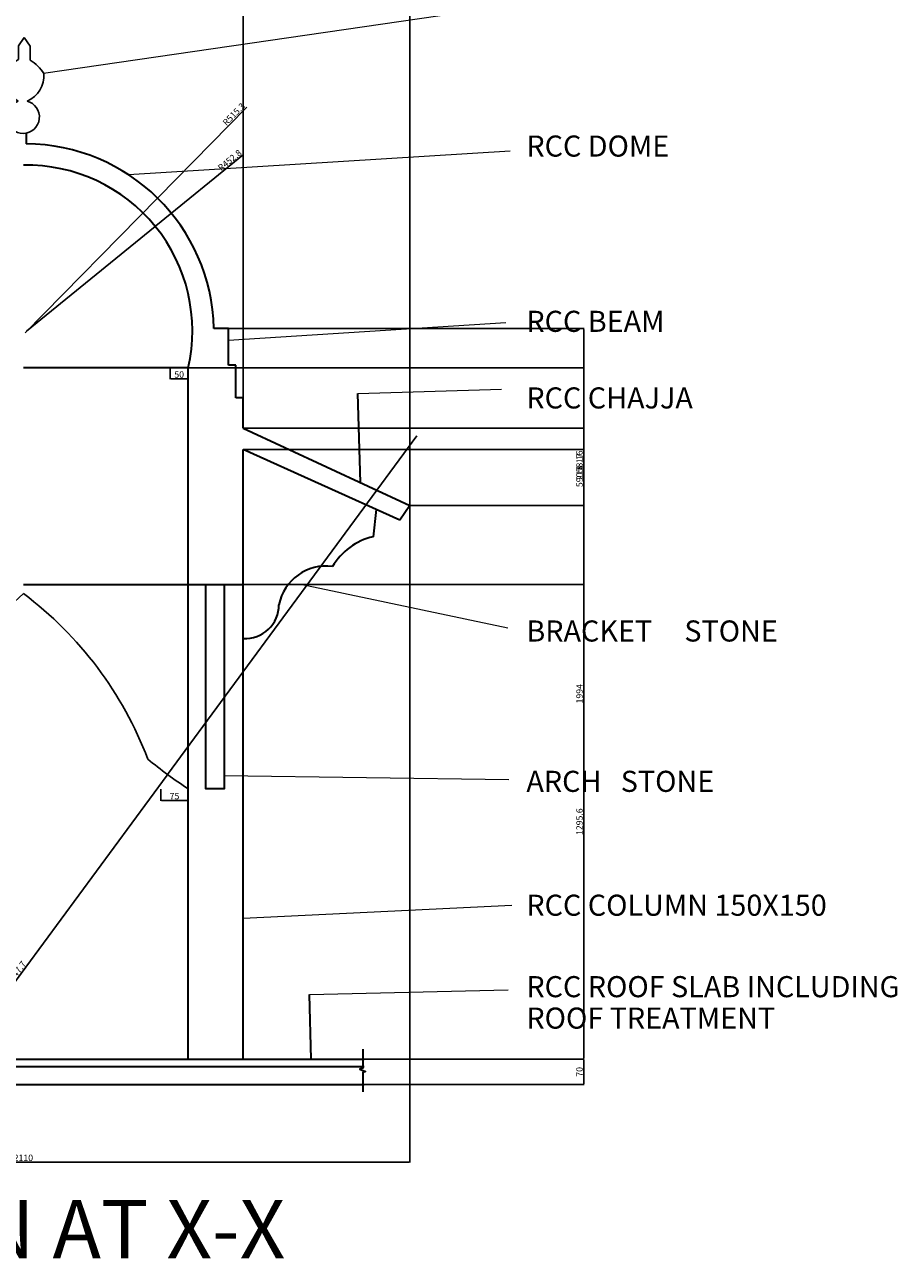
# Model space of a CAD drawing. Units: millimetres. Extents: x 498 to 8860, y -426 to 8717.
# Tile 6 of 9: x 1798 to 4180, y 3606 to 6976. Entities that reach past the tile are written whole.
import ezdxf

# ---------------------------------------------------------------- set-up
doc = ezdxf.new("R2010")
doc.units = ezdxf.units.MM
for name, color, linetype, lineweight in [('A-ANNO-DIMS', 2, 'Continuous', 18), ('A-ANNO-TEXT', 3, 'Continuous', 18), ('A-DETL', 7, 'Continuous', 25), ('A-SECT', 7, 'Continuous', 35)]:
    doc.layers.add(name, color=color, linetype=linetype, lineweight=lineweight)
doc.styles.get("Standard").update_dxf_attribs({"font": 'arial.ttf'})
doc.dimstyles.new('ISO-25', dxfattribs={"dimtxt": 17.5, "dimasz": 2.5, "dimexe": 1.25, "dimexo": 0.625, "dimtad": 1, "dimdec": 0, "dimtxsty": 'Standard', "dimcen": 2.5, "dimadec": 0, "dimazin": 0, "dimtfac": 1, "dimtdec": 0, "dimtmove": 0, "dimatfit": 3, "dimfxl": 1, "dimarcsym": 0})

# ---------------------------------------------------------------- blocks, each defined once
blk = doc.blocks.new('*D30')
at = {"layer": 'A-ANNO-DIMS', "color": 0, "lineweight": -2, "transparency": 16777216}
for p, q in [((2195, 6038.9), (2195, 6008.7)), ((2244.7, 6038.9), (2244.7, 6008.7)), ((2242.2, 6010), (2197.5, 6010))]:
    blk.add_line(p, q, dxfattribs=at)
at = {"layer": 'A-ANNO-DIMS', "color": 0, "transparency": 16777216}
for points in [[(2197.5, 6010.4), (2197.5, 6009.6), (2195, 6010)], [(2242.2, 6010.4), (2242.2, 6009.6), (2244.7, 6010)]]:
    blk.add_solid(points, dxfattribs=at)
at = {"layer": 'Defpoints', "color": 0, "transparency": 16777216}
for p in [(2195, 6039.5), (2244.7, 6039.5), (2195, 6010)]:
    blk.add_point(p, dxfattribs=at)
at = {"layer": 'A-ANNO-DIMS', "color": 0, "transparency": 16777216, "insert": (2219.9, 6019.5), "char_height": 17.5, "attachment_point": 5}
blk.add_mtext('50', dxfattribs=at)
blk = doc.blocks.new('*D33')
at = {"layer": 'A-ANNO-DIMS', "color": 0, "lineweight": -2, "transparency": 16777216}
for p, q in [((2169.5, 4890.1), (2169.5, 4857.7)), ((2244.7, 4889.9), (2244.7, 4857.7)), ((2242.2, 4858.9), (2172, 4858.9))]:
    blk.add_line(p, q, dxfattribs=at)
at = {"layer": 'A-ANNO-DIMS', "color": 0, "transparency": 16777216}
for points in [[(2172, 4859.3), (2172, 4858.5), (2169.5, 4858.9)], [(2242.2, 4859.3), (2242.2, 4858.5), (2244.7, 4858.9)]]:
    blk.add_solid(points, dxfattribs=at)
at = {"layer": 'Defpoints', "color": 0, "transparency": 16777216}
for p in [(2169.5, 4890.7), (2244.7, 4890.6), (2169.5, 4858.9)]:
    blk.add_point(p, dxfattribs=at)
at = {"layer": 'A-ANNO-DIMS', "color": 0, "transparency": 16777216, "insert": (2207.1, 4868.4), "char_height": 17.5, "attachment_point": 5}
blk.add_mtext('75', dxfattribs=at)
blk = doc.blocks.new('FINIAL-BRASS')
for p, q in [((41.3, 239), (57, 261.6)), ((41.3, 202), (41.3, 239)), ((57, 261.6), (73.3, 238.5)), ((73.3, 199.9), (73.3, 238.5))]:
    blk.add_line(p, q)
for centre, radius, start, end in [((108.5, 89), 131.5, 120.7656, 145.5289), ((18.2, 106.2), 108.7, 31.7357, 59.5088), ((81.5, 158.5), 81.5, 176.5528, 239.9655), ((34.6, 158.5), 76.2, 293.2182, 3.7332), ((53.5, 44.9), 44.9, 106.5437, 75.6662)]:
    blk.add_arc(centre, radius, start, end)
blk = doc.blocks.new('BRACKET-STONE')
for centre, radius, start, end in [((1183.8, -291.1), 1104.6, 131.6209, 159.0769), ((-158.8, -276), 1013.9, 20.7397, 53.0882), ((-446.2, 819.4), 933, 298.5683, 309.875), ((1523.8, 965), 1147.7, 230.2129, 237.0762)]:
    blk.add_arc(centre, radius, start, end)
blk = doc.blocks.new('*D43')
at = {"layer": 'A-ANNO-DIMS', "color": 0, "lineweight": -2, "transparency": 16777216}
for p, q in [((739.8, 5663.4), (739.8, 3870.5)), ((2849.6, 5663.4), (2849.6, 3870.5)), ((742.3, 3871.8), (2847.1, 3871.8))]:
    blk.add_line(p, q, dxfattribs=at)
at = {"layer": 'A-ANNO-DIMS', "color": 0, "transparency": 16777216}
for points in [[(742.3, 3872.2), (742.3, 3871.3), (739.8, 3871.8)], [(2847.1, 3872.2), (2847.1, 3871.3), (2849.6, 3871.8)]]:
    blk.add_solid(points, dxfattribs=at)
at = {"layer": 'Defpoints', "color": 0, "transparency": 16777216}
for p in [(739.8, 5664), (2849.6, 5664), (2849.6, 3871.8)]:
    blk.add_point(p, dxfattribs=at)
at = {"layer": 'A-ANNO-DIMS', "color": 0, "transparency": 16777216, "insert": (1794.7, 3881.3), "char_height": 17.5, "attachment_point": 5}
blk.add_mtext('2110', dxfattribs=at)
blk = doc.blocks.new('*D45')
at = {"layer": 'A-ANNO-DIMS', "color": 0, "lineweight": -2, "transparency": 16777216}
for p, q in [((2395.4, 5448.8), (3325.4, 5448.8)), ((3324.2, 4155.7), (3324.2, 5446.3)), ((2395.4, 4153.2), (3325.4, 4153.2))]:
    blk.add_line(p, q, dxfattribs=at)
at = {"layer": 'A-ANNO-DIMS', "color": 0, "transparency": 16777216}
for points in [[(3323.8, 5446.3), (3324.6, 5446.3), (3324.2, 5448.8)], [(3323.8, 4155.7), (3324.6, 4155.7), (3324.2, 4153.2)]]:
    blk.add_solid(points, dxfattribs=at)
at = {"layer": 'Defpoints', "color": 0, "transparency": 16777216}
for p in [(2394.7, 5448.8), (3324.2, 5448.8), (2394.7, 4153.2)]:
    blk.add_point(p, dxfattribs=at)
at = {"layer": 'A-ANNO-DIMS', "color": 0, "transparency": 16777216, "insert": (3314.6, 4801), "char_height": 17.5, "attachment_point": 5, "rotation": 90}
blk.add_mtext('1295.6', dxfattribs=at)
blk = doc.blocks.new('*D46')
at = {"layer": 'A-ANNO-DIMS', "color": 0, "lineweight": -2, "transparency": 16777216}
for p, q in [((2245.4, 6039.5), (3325.4, 6039.5)), ((3324.2, 5451.3), (3324.2, 6037)), ((2245.4, 5448.8), (3325.4, 5448.8))]:
    blk.add_line(p, q, dxfattribs=at)
at = {"layer": 'A-ANNO-DIMS', "color": 0, "transparency": 16777216}
for points in [[(3323.8, 6037), (3324.6, 6037), (3324.2, 6039.5)], [(3323.8, 5451.3), (3324.6, 5451.3), (3324.2, 5448.8)]]:
    blk.add_solid(points, dxfattribs=at)
at = {"layer": 'Defpoints', "color": 0, "transparency": 16777216}
for p in [(2244.7, 6039.5), (3324.2, 6039.5), (2244.7, 5448.8)]:
    blk.add_point(p, dxfattribs=at)
at = {"layer": 'A-ANNO-DIMS', "color": 0, "transparency": 16777216, "insert": (3314.6, 5744.1), "char_height": 17.5, "attachment_point": 5, "rotation": 90}
blk.add_mtext('590.8', dxfattribs=at)
blk = doc.blocks.new('*D47')
at = {"layer": 'A-ANNO-DIMS', "color": 0, "lineweight": -2, "transparency": 16777216}
for p, q in [((2315.4, 6147.2), (3325.4, 6147.2)), ((3324.2, 4155.7), (3324.2, 6144.7)), ((2395.4, 4153.2), (3325.4, 4153.2))]:
    blk.add_line(p, q, dxfattribs=at)
at = {"layer": 'A-ANNO-DIMS', "color": 0, "transparency": 16777216}
for points in [[(3323.8, 6144.7), (3324.6, 6144.7), (3324.2, 6147.2)], [(3323.8, 4155.7), (3324.6, 4155.7), (3324.2, 4153.2)]]:
    blk.add_solid(points, dxfattribs=at)
at = {"layer": 'Defpoints', "color": 0, "transparency": 16777216}
for p in [(2314.7, 6147.2), (3324.2, 6147.2), (2394.7, 4153.2)]:
    blk.add_point(p, dxfattribs=at)
at = {"layer": 'A-ANNO-DIMS', "color": 0, "transparency": 16777216, "insert": (3314.6, 5150.2), "char_height": 17.5, "attachment_point": 5, "rotation": 90}
blk.add_mtext('1994', dxfattribs=at)
blk = doc.blocks.new('*D48')
at = {"layer": 'A-ANNO-DIMS', "color": 0, "lineweight": -2, "transparency": 16777216}
for p, q in [((2395.4, 5875.2), (3325.4, 5875.2)), ((3324.2, 5872.7), (3324.2, 5819.5)), ((2395.4, 5817), (3325.4, 5817)), ((3324.2, 5817), (3324.2, 5754.2))]:
    blk.add_line(p, q, dxfattribs=at)
at = {"layer": 'A-ANNO-DIMS', "color": 0, "transparency": 16777216}
for points in [[(3323.8, 5872.7), (3324.6, 5872.7), (3324.2, 5875.2)], [(3323.8, 5819.5), (3324.6, 5819.5), (3324.2, 5817)]]:
    blk.add_solid(points, dxfattribs=at)
at = {"layer": 'Defpoints', "color": 0, "transparency": 16777216}
for p in [(2394.7, 5875.2), (2394.7, 5817), (3324.2, 5817)]:
    blk.add_point(p, dxfattribs=at)
at = {"layer": 'A-ANNO-DIMS', "color": 0, "transparency": 16777216, "insert": (3314.6, 5784.4), "char_height": 17.5, "attachment_point": 5, "rotation": 90}
blk.add_mtext('58.16', dxfattribs=at)
blk = doc.blocks.new('*D49')
at = {"layer": 'A-ANNO-DIMS', "color": 0, "lineweight": -2, "transparency": 16777216}
for p, q in [((2394.7, 5875.8), (2394.7, 7224.4)), ((2397.2, 7223.1), (2847.1, 7223.1)), ((2849.6, 5664.6), (2849.6, 7224.4))]:
    blk.add_line(p, q, dxfattribs=at)
at = {"layer": 'A-ANNO-DIMS', "color": 0, "transparency": 16777216}
for points in [[(2397.2, 7223.5), (2397.2, 7222.7), (2394.7, 7223.1)], [(2847.1, 7223.5), (2847.1, 7222.7), (2849.6, 7223.1)]]:
    blk.add_solid(points, dxfattribs=at)
at = {"layer": 'Defpoints', "color": 0, "transparency": 16777216}
for p in [(2849.6, 7223.1), (2394.7, 5875.2), (2849.6, 5664)]:
    blk.add_point(p, dxfattribs=at)
at = {"layer": 'A-ANNO-DIMS', "color": 0, "transparency": 16777216, "insert": (2622.2, 7232.7), "char_height": 17.5, "attachment_point": 5}
blk.add_mtext('454.9', dxfattribs=at)
blk = doc.blocks.new('*D50')
at = {"layer": 'A-ANNO-DIMS', "color": 0, "lineweight": -2, "transparency": 16777216}
for p, q in [((2395.4, 5875.2), (3325.4, 5875.2)), ((3324.2, 5872.7), (3324.2, 5666.5)), ((2850.3, 5664), (3325.4, 5664))]:
    blk.add_line(p, q, dxfattribs=at)
at = {"layer": 'A-ANNO-DIMS', "color": 0, "transparency": 16777216}
for points in [[(3323.8, 5872.7), (3324.6, 5872.7), (3324.2, 5875.2)], [(3323.8, 5666.5), (3324.6, 5666.5), (3324.2, 5664)]]:
    blk.add_solid(points, dxfattribs=at)
at = {"layer": 'Defpoints', "color": 0, "transparency": 16777216}
for p in [(2394.7, 5875.2), (2849.6, 5664), (3324.2, 5664)]:
    blk.add_point(p, dxfattribs=at)
at = {"layer": 'A-ANNO-DIMS', "color": 0, "transparency": 16777216, "insert": (3314.8, 5769.6), "char_height": 17.5, "attachment_point": 5, "rotation": 90}
blk.add_mtext('211.17', dxfattribs=at)
blk = doc.blocks.new('*D51')
at = {"layer": 'A-ANNO-DIMS', "color": 0, "lineweight": -2, "transparency": 16777216}
for p, q in [((2725.4, 4153.2), (3325.4, 4153.2)), ((3324.2, 4150.7), (3324.2, 4085.7)), ((2725.4, 4083.2), (3325.4, 4083.2))]:
    blk.add_line(p, q, dxfattribs=at)
at = {"layer": 'A-ANNO-DIMS', "color": 0, "transparency": 16777216}
for points in [[(3323.8, 4150.7), (3324.6, 4150.7), (3324.2, 4153.2)], [(3323.8, 4085.7), (3324.6, 4085.7), (3324.2, 4083.2)]]:
    blk.add_solid(points, dxfattribs=at)
at = {"layer": 'Defpoints', "color": 0, "transparency": 16777216}
for p in [(2724.7, 4153.2), (2724.7, 4083.2), (3324.2, 4083.2)]:
    blk.add_point(p, dxfattribs=at)
at = {"layer": 'A-ANNO-DIMS', "color": 0, "transparency": 16777216, "insert": (3314.6, 4118.2), "char_height": 17.5, "attachment_point": 5, "rotation": 90}
blk.add_mtext('70', dxfattribs=at)
blk = doc.blocks.new('*D74')
at = {"layer": 'A-ANNO-DIMS', "color": 0, "lineweight": -2, "transparency": 16777216}
for p, q in [((2404.4, 6751.2), (2162.5, 6505)), ((1799.6, 6135.6), (2160.7, 6503.2))]:
    blk.add_line(p, q, dxfattribs=at)
at = {"layer": 'A-ANNO-DIMS', "color": 0, "transparency": 16777216}
blk.add_solid([(2162.2, 6505.3), (2162.7, 6504.7), (2160.7, 6503.2)], dxfattribs=at)
at = {"layer": 'Defpoints', "color": 0, "transparency": 16777216}
for p in [(2160.7, 6503.2), (1799.6, 6135.6)]:
    blk.add_point(p, dxfattribs=at)
at = {"layer": 'A-ANNO-DIMS', "color": 0, "transparency": 16777216, "insert": (2370.6, 6730.4), "char_height": 17.5, "attachment_point": 5, "rotation": 45.5059}
blk.add_mtext('R515.3', dxfattribs=at)
blk = doc.blocks.new('*D75')
at = {"layer": 'A-ANNO-DIMS', "color": 0, "lineweight": -2, "transparency": 16777216}
for p, q in [((2395.3, 6621.7), (2156.5, 6427.6)), ((1803.3, 6140.3), (2154.6, 6426))]:
    blk.add_line(p, q, dxfattribs=at)
at = {"layer": 'A-ANNO-DIMS', "color": 0, "transparency": 16777216}
blk.add_solid([(2156.3, 6427.9), (2156.8, 6427.3), (2154.6, 6426)], dxfattribs=at)
at = {"layer": 'Defpoints', "color": 0, "transparency": 16777216}
for p in [(2154.6, 6426), (1803.3, 6140.3)]:
    blk.add_point(p, dxfattribs=at)
at = {"layer": 'A-ANNO-DIMS', "color": 0, "transparency": 16777216, "insert": (2359.3, 6604.8), "char_height": 17.5, "attachment_point": 5, "rotation": 39.1178}
blk.add_mtext('R452.8', dxfattribs=at)
blk = doc.blocks.new('*D76')
at = {"layer": 'A-ANNO-DIMS', "color": 0, "lineweight": -2, "transparency": 16777216}
for p, q in [((2868.5, 5853.9), (2188.2, 4929.6)), ((1753.1, 4338.5), (2186.7, 4927.6))]:
    blk.add_line(p, q, dxfattribs=at)
at = {"layer": 'A-ANNO-DIMS', "color": 0, "transparency": 16777216}
blk.add_solid([(2186.4, 4927.8), (2187.1, 4927.3), (2188.2, 4929.6)], dxfattribs=at)
at = {"layer": 'Defpoints', "color": 0, "transparency": 16777216}
for p in [(2868.5, 5853.9), (2188.2, 4929.6)]:
    blk.add_point(p, dxfattribs=at)
at = {"layer": 'A-ANNO-DIMS', "color": 0, "transparency": 16777216, "insert": (1772.4, 4380.6), "char_height": 17.5, "attachment_point": 5, "rotation": 53.6461}
blk.add_mtext('R1147.7', dxfattribs=at)

msp = doc.modelspace()

# ---------------------------------------------------------------- linework, layer by layer
at = {"layer": 'A-ANNO-TEXT'}
for p, q in [((2081.16, 6567.175), (3122.821, 6631.816)), ((2354.726, 6115.745), (3111.023, 6163.21)), ((2707.096, 5969.553), (3099.478, 5981.733)), ((2552.178, 5449.241), (3116.865, 5330.088)), ((2342.353, 4927.161), (3119.838, 4915.994)), ((2394.726, 4538.083), (3127.724, 4573.133)), ((2575.958, 4329.528), (3117.407, 4341.91))]:
    msp.add_line(p, q, dxfattribs=at)
msp.add_lwpolyline([(1849.694, 6844.528), (3132.176, 7031.12)], dxfattribs=at)
at = {"layer": 'A-SECT'}
for p, q in [((1802.162, 6680.333), (1802.162, 6650.916)), ((2354.726, 6147.245), (2314.726, 6147.245)), ((2354.726, 6047.245), (2354.726, 6147.245)), ((2244.726, 6039.541), (1794.726, 6039.541)), ((2244.726, 5448.755), (2244.726, 6039.541)), ((2374.726, 6047.245), (2354.726, 6047.245)), ((2374.726, 5957.887), (2374.726, 6047.245)), ((2714.636, 5726.663), (2707.096, 5969.553)), ((2394.726, 5957.887), (2374.726, 5957.887)), ((2394.726, 5875.163), (2394.726, 5957.887)), ((2394.726, 5875.163), (2849.644, 5663.993)), ((2394.726, 5448.755), (2394.726, 5817.007)), ((2822.299, 5623.74), (2394.726, 5817.007)), ((2849.644, 5663.993), (2822.299, 5623.74)), ((2757.051, 5653.233), (2749.118, 5578.673)), ((1794.726, 5448.755), (2394.726, 5448.755)), ((2244.726, 4153.169), (2244.726, 5448.755)), ((2394.726, 4153.169), (2394.726, 5448.755)), ((2579.991, 4153.169), (2575.958, 4329.528)), ((864.726, 4153.169), (2724.726, 4153.169)), ((864.726, 4133.169), (2724.726, 4133.169)), ((864.726, 4083.169), (2724.726, 4083.169))]:
    msp.add_line(p, q, dxfattribs=at)
msp.add_lwpolyline([(2293.009, 5448.755), (2342.353, 5448.755), (2342.353, 4890.556), (2293.009, 4890.556)], close=True, dxfattribs=at)
msp.add_lwpolyline([(2721.018, 4180.433), (2721.018, 4127.866), (2713.259, 4125.041), (2728.777, 4119.393), (2721.018, 4116.569), (2721.018, 4063.756)], dxfattribs=at)
for centre, radius, start, end in [((1799.566, 6135.632), 515.29, 1.291337, 89.711428), ((1803.318, 6140.339), 452.771, 347.13675, 91.087286), ((2787.134, 5410.667), 172.253, 102.750062, 149.710295), ((2620.732, 5367.687), 131.056, 82.254004, 168.811873), ((2400.225, 5393.116), 91.941, 266.570991, 360)]:
    msp.add_arc(centre, radius, start, end, dxfattribs=at)

# ---------------------------------------------------------------- block references
at = {"layer": 'A-DETL'}
for name, p in [('FINIAL-BRASS', (1740.051, 6679.509)), ('BRACKET-STONE', (1344.726, 4888.954))]:
    msp.add_blockref(name, p, dxfattribs=at)

# ---------------------------------------------------------------- texts
at = {"layer": 'A-ANNO-TEXT'}
for s, height, p in [('RCC DOME', 57.5404, (3167.376, 6616.418)), ('RCC BEAM', 57.5404, (3167.376, 6138.023)), ('RCC CHAJJA', 57.5404, (3167.376, 5928.899)), ('BRACKET     STONE', 57.54038, (3167.376, 5292.736)), ('ARCH   STONE', 57.54038, (3167.376, 4882.363)), ('RCC COLUMN 150X150 ', 57.54038, (3167.376, 4544.23)), ('RCC ROOF SLAB INCLUDING', 57.54038, (3167.376, 4321.904)), ('ROOF TREATMENT', 57.54038, (3167.376, 4236.094)), ('SECTION AT X-X', 159.20004, (917.853, 3609.29))]:
    msp.add_text(s, height=height, dxfattribs=at).set_placement(p)

# ---------------------------------------------------------------- dimensions: what is measured, and where the dimension line sits
at = {"layer": 'A-ANNO-DIMS'}
for base, p1, p2, override, picture, middle in [((2849.644, 7223.12), (2394.726, 5875.163), (2849.644, 5663.993), {"dimdec": 1, "dimlfac": 1, "dimrnd": 0, "dimzin": 0, "dimdsep": 46, "dimlunit": 2}, '*D49', (2622.185, 7232.68)), ((2194.985, 6009.99), (2244.726, 6039.541), (2194.985, 6039.541), {"dimclrd": 0, "dimclre": 0, "dimclrt": 0}, '*D30', (2219.855, 6019.55)), ((2849.644, 3871.756), (739.808, 5663.993), (2849.644, 5663.993), {"dimdec": 0, "dimlfac": 1, "dimrnd": 0, "dimzin": 0, "dimdsep": 46, "dimlunit": 2}, '*D43', (1794.726, 3881.316)), ((2169.469, 4858.902), (2244.726, 4890.556), (2169.469, 4890.723), {"dimclrd": 0, "dimclre": 0, "dimclrt": 0}, '*D33', (2207.097, 4868.426))]:
    dim = msp.add_linear_dim(base=base, p1=p1, p2=p2, dimstyle='ISO-25', override=override, dxfattribs=at)
    dim.commit()
    dim.dimension.update_dxf_attribs({"geometry": picture, "text_midpoint": middle})
for center, mpoint, picture, middle in [((1799.566, 6135.632), (2160.7, 6503.2), '*D74', (2377.381, 6723.741)), ((1803.318, 6140.339), (2154.6, 6426), '*D75', (2365.37, 6597.397)), ((2868.528, 5853.93), (2188.204, 4929.605), '*D76', (1780.009, 4375.01))]:
    dim = msp.add_radius_dim(center=center, mpoint=mpoint, dimstyle='ISO-25', override={"dimdec": 1, "dimlfac": 1, "dimrnd": 0, "dimzin": 0, "dimdsep": 46, "dimlunit": 2}, dxfattribs=at)
    dim.commit()
    dim.dimension.update_dxf_attribs({"geometry": picture, "text_midpoint": middle, "dimtype": 164})
for base, p1, p2, override, picture, middle in [((3324.176, 6147.245), (2394.726, 4153.169), (2314.726, 6147.245), {"dimdec": 0, "dimlfac": 1, "dimrnd": 0, "dimzin": 0, "dimdsep": 46, "dimlunit": 2}, '*D47', (3314.616, 5150.207)), ((3324.176, 6039.541), (2244.726, 5448.755), (2244.726, 6039.541), {"dimdec": 1, "dimlfac": 1, "dimrnd": 0, "dimzin": 0, "dimdsep": 46, "dimlunit": 2}, '*D46', (3314.616, 5744.148)), ((3324.176, 5817.007), (2394.726, 5875.163), (2394.726, 5817.007), {"dimdec": 2, "dimlfac": 1, "dimrnd": 0, "dimzin": 0, "dimdsep": 46, "dimlunit": 2}, '*D48', (3314.616, 5784.361)), ((3324.176, 5663.993), (2394.726, 5875.163), (2849.644, 5663.993), {"dimdec": 2, "dimlfac": 1, "dimrnd": 0, "dimzin": 0, "dimdsep": 46, "dimlunit": 2}, '*D50', (3314.766, 5769.578)), ((3324.176, 5448.755), (2394.726, 4153.169), (2394.726, 5448.755), {"dimdec": 1, "dimlfac": 1, "dimrnd": 0, "dimzin": 0, "dimdsep": 46, "dimlunit": 2}, '*D45', (3314.616, 4800.962)), ((3324.176, 4083.169), (2724.726, 4153.169), (2724.726, 4083.169), {"dimdec": 0, "dimlfac": 1, "dimrnd": 0, "dimzin": 0, "dimdsep": 46, "dimlunit": 2}, '*D51', (3314.616, 4118.169))]:
    dim = msp.add_linear_dim(base=base, p1=p1, p2=p2, angle=90, dimstyle='ISO-25', override=override, dxfattribs=at)
    dim.commit()
    dim.dimension.update_dxf_attribs({"geometry": picture, "text_midpoint": middle})

doc.saveas('drawing.dxf')
